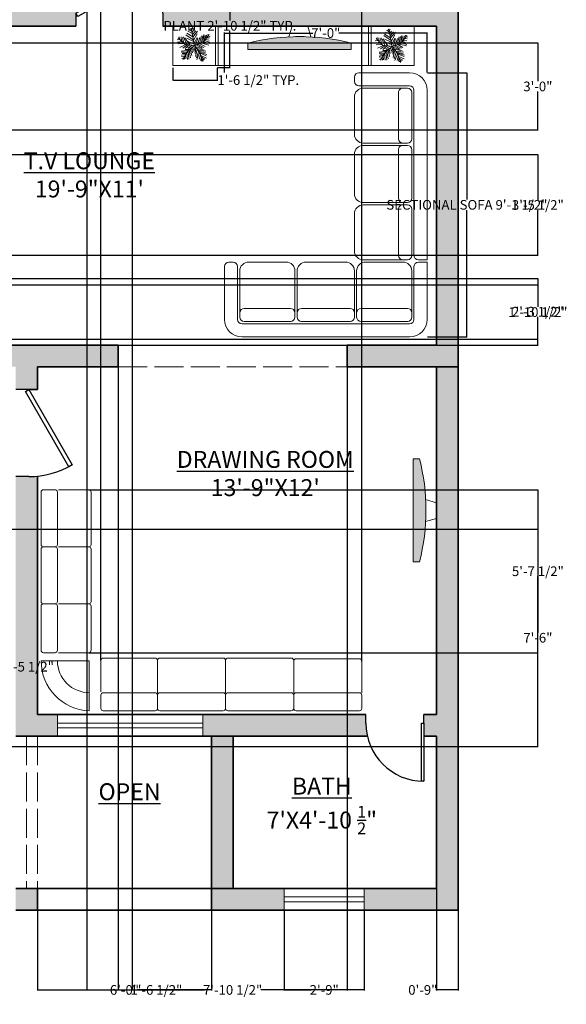
# Model space of a CAD drawing. Units: inches. Extents: x -37 to 408, y -619 to 75.
# Tile 3 of 4: x 182 to 408, y -619 to -212. Entities that reach past the tile are written whole.
import ezdxf

# ---------------------------------------------------------------- set-up
doc = ezdxf.new("R2010")
doc.units = ezdxf.units.IN
doc.header["$MEASUREMENT"] = 0
doc.linetypes.add('ACAD_ISO02W100', pattern=[15, 12, -3])
for name, color, linetype, lineweight in [('A-ANNO-DIMS', 2, 'Continuous', 18), ('A-AREA-IDEN', 7, 'Continuous', 25), ('A-DOOR', 4, 'Continuous', 25), ('A-EQPM', 9, 'Continuous', 18), ('A-FLOR-CASE', 8, 'Continuous', 18), ('A-FURN', 8, 'Continuous', 18), ('A-GLAZ', 4, 'Continuous', 18), ('A-WALL', 7, 'Continuous', 35), ('A-WALL-OVHD', 7, 'ACAD_ISO02W100', 18), ('A-WALL-PATT', 16, 'Continuous', 13), ('tree', 3, 'Continuous', 13)]:
    doc.layers.add(name, color=color, linetype=linetype, lineweight=lineweight)
doc.styles.get("Standard").update_dxf_attribs({"font": 'arial.ttf'})
doc.dimstyles.get("Standard").update_dxf_attribs({"dimtxt": 4, "dimasz": 0.18, "dimexe": 0.18, "dimexo": 0.0625, "dimgap": 0.09, "dimtad": 0, "dimtih": 1, "dimtoh": 1, "dimdec": 1, "dimzin": 0, "dimdsep": 46, "dimlunit": 4, "dimtxsty": 'Standard', "dimcen": 0.09, "dimadec": 0, "dimazin": 0, "dimtfac": 1, "dimtdec": 1, "dimtofl": 0, "dimtmove": 0, "dimatfit": 3, "dimfxl": 1, "dimtolj": 1, "dimtzin": 0, "dimarcsym": 0})

# ---------------------------------------------------------------- blocks, each defined once
blk = doc.blocks.new('*U2')
for p, q in [((0, 0), (0, -6)), ((40, 0), (40, -6))]:
    blk.add_line(p, q)
blk.add_lwpolyline([(0, 0), (34.64, 20), (35.52, 18.48), (0.87, -1.52)], close=True)
blk.add_arc((0, 0), 40, 0, 30)
blk = doc.blocks.new('*U3')
for p, q in [((0, 0), (0, -6)), ((40, 0), (40, -6))]:
    blk.add_line(p, q)
blk.add_lwpolyline([(0, 0), (0, 40), (1.75, 40), (1.75, 0)], close=True)
blk.add_arc((0, 0), 40, 0, 90)
blk = doc.blocks.new('A$C2AFA021D')
for p, q in [((0.8, 2.3), (0.2, 2.3)), ((0.85, 2.2), (0.85, 2.25)), ((0.2, 2.15), (0.8, 2.15)), ((0.225, 2.125), (0.275, 2.125)), ((0.75, 2.125), (0.275, 2.125)), ((0, 2.1), (0, 0.2)), ((0.15, 0.2), (0.15, 2.1)), ((0.175, 1.55), (0.175, 2.075)), ((0.325, 2.075), (0.325, 1.55)), ((0.85, 1.6), (0.85, 2.025)), ((0.275, 1.5), (0.225, 1.5)), ((0.225, 1.475), (0.275, 1.475)), ((0.275, 1.5), (0.75, 1.5)), ((0.75, 1.475), (0.275, 1.475)), ((0.175, 0.875), (0.175, 1.425)), ((0.325, 1.425), (0.325, 0.875)), ((0.85, 0.925), (0.85, 1.375)), ((0.275, 0.825), (0.225, 0.825)), ((0.225, 0.8), (0.275, 0.8)), ((0.275, 0.825), (0.75, 0.825)), ((0.75, 0.8), (0.275, 0.8)), ((0.975, 0.825), (1.4, 0.825)), ((1.625, 0.825), (2.075, 0.825)), ((2.3, 0.825), (2.725, 0.825)), ((2.9, 0.825), (2.95, 0.825)), ((0.175, 0.225), (0.175, 0.75)), ((0.325, 0.75), (0.325, 0.225)), ((0.85, 0.275), (0.85, 0.7)), ((0.875, 0.275), (0.875, 0.725)), ((1.5, 0.725), (1.5, 0.275)), ((1.525, 0.275), (1.525, 0.725)), ((2.175, 0.725), (2.175, 0.275)), ((2.2, 0.275), (2.2, 0.725)), ((2.825, 0.725), (2.825, 0.275)), ((2.85, 0.2), (2.85, 0.775)), ((3, 0.775), (3, 0.2)), ((0.875, 0.275), (0.875, 0.225)), ((1.45, 0.325), (0.925, 0.325)), ((1.5, 0.225), (1.5, 0.275)), ((1.525, 0.275), (1.525, 0.225)), ((2.125, 0.325), (1.575, 0.325)), ((2.175, 0.225), (2.175, 0.275)), ((2.2, 0.275), (2.2, 0.225)), ((2.775, 0.325), (2.25, 0.325)), ((2.825, 0.225), (2.825, 0.275)), ((0.8, 0.15), (0.2, 0.15)), ((0.275, 0.175), (0.225, 0.175)), ((0.275, 0.175), (0.75, 0.175)), ((0.925, 0.175), (1.45, 0.175)), ((0.925, 0.15), (2.8, 0.15)), ((1.575, 0.175), (2.125, 0.175)), ((2.25, 0.175), (2.775, 0.175)), ((0.85, 0), (0.85, 0.1)), ((0.875, 0.1), (0.875, 0)), ((0.2, 0), (0.85, 0)), ((2.8, 0), (0.875, 0))]:
    blk.add_line(p, q)
for centre, radius, start, end in [((0.2, 2.1), 0.2, 90, 180), ((0.8, 2.25), 0.05, 0, 90), ((0.2, 2.1), 0.05, 90, 180), ((0.225, 2.075), 0.05, 90, 180), ((0.275, 2.075), 0.05, 0, 90), ((0.75, 2.025), 0.1, 0, 90), ((0.8, 2.2), 0.05, 270, 0), ((0.75, 1.6), 0.1, 270, 0), ((0.225, 1.55), 0.05, 180, 270), ((0.225, 1.425), 0.05, 90, 180), ((0.275, 1.55), 0.05, 270, 0), ((0.275, 1.425), 0.05, 0, 90), ((0.75, 1.375), 0.1, 360, 90), ((0.75, 0.925), 0.1, 270, 0), ((0.225, 0.875), 0.05, 180, 270), ((0.225, 0.75), 0.05, 90, 180), ((0.275, 0.875), 0.05, 270, 0), ((0.275, 0.75), 0.05, 0, 90), ((0.75, 0.7), 0.1, 0, 90), ((0.975, 0.725), 0.1, 90, 180), ((1.4, 0.725), 0.1, 0, 90), ((1.625, 0.725), 0.1, 90, 180), ((2.075, 0.725), 0.1, 0, 90), ((2.3, 0.725), 0.1, 90, 180), ((2.725, 0.725), 0.1, 0, 90), ((2.9, 0.775), 0.05, 90, 180), ((2.95, 0.775), 0.05, 0, 90), ((0.225, 0.225), 0.05, 180, 270), ((0.275, 0.225), 0.05, 270, 0), ((0.75, 0.275), 0.1, 270, 0), ((0.925, 0.275), 0.05, 90, 180), ((0.925, 0.225), 0.05, 180, 270), ((1.45, 0.275), 0.05, 360, 90), ((1.45, 0.225), 0.05, 270, 0), ((1.575, 0.275), 0.05, 90, 180), ((1.575, 0.225), 0.05, 180, 270), ((2.125, 0.275), 0.05, 360, 90), ((2.125, 0.225), 0.05, 270, 0), ((2.25, 0.275), 0.05, 90, 180), ((2.25, 0.225), 0.05, 180, 270), ((2.775, 0.275), 0.05, 360, 90), ((2.775, 0.225), 0.05, 270, 0), ((0.2, 0.2), 0.2, 180, 270), ((0.2, 0.2), 0.05, 180, 270), ((0.8, 0.1), 0.05, 0, 90), ((0.925, 0.1), 0.05, 90, 180), ((2.8, 0.2), 0.2, 270, 0), ((2.8, 0.2), 0.05, 270, 0)]:
    blk.add_arc(centre, radius, start, end)
blk = doc.blocks.new('Trees - Imperial')
for p, q in [((-3.665, 19.273), (-27.574, 35.527)), ((-5.114, 28.097), (-24.676, 40.636)), ((-7.288, 39.707), (-21.778, 46.673)), ((-8.737, 47.138), (-17.069, 52.711)), ((-10.186, 53.64), (-13.084, 55.962)), ((0, 0), (-10.5, 57)), ((-9.099, 51.782), (-6.563, 55.962)), ((-7.65, 43.423), (-2.578, 49.46)), ((-5.839, 35.992), (4.667, 48.067)), ((-5.114, 27.632), (10.463, 46.673)), ((-2.941, 16.486), (8.652, 37.85)), ((22.055, 7.198), (27.489, 32.277)), ((27, 9), (48, 36)), ((27.127, 9.056), (31.112, 35.992)), ((35.096, 32.741), (37.27, 22.524)), ((38.719, 34.134), (41.979, 28.561)), ((44.153, 36.456), (45.239, 32.741)), ((-47.498, 19.737), (-55.83, 18.344)), ((-40.615, 13.7), (-55.105, 10.913)), ((-31.5, 4.5), (-52.5, 25.5)), ((-33.37, 6.269), (-52.207, 5.34)), ((-48.585, 21.131), (-49.309, 29.026)), ((-28.299, 3.483), (-47.86, -5.805)), ((-43.513, 28.561), (-42.427, 15.558)), ((-38.442, 26.239), (-34.819, 7.663)), ((-21.416, 3.018), (-38.079, -8.128)), ((-35.544, 28.097), (-24.314, 3.947)), ((0, 0), (-31.5, 4.5)), ((-14.533, 2.09), (-30.834, 25.31)), ((-15.982, 2.09), (-30.11, -9.521)), ((-24.314, 23.917), (-2.941, 13.7)), ((0, 0), (-22.5, -19.5)), ((-6.563, 1.161), (-21.416, -8.128)), ((-20.691, 13.7), (-1.129, 4.876)), ((-1.129, 6.734), (9.014, 26.704)), ((0, 0), (27, 9)), ((0, 0), (18, -22.5)), ((3.942, 1.625), (11.187, 24.381)), ((6.478, 1.625), (26.04, -8.592)), ((10.101, 3.483), (17.708, 26.239)), ((11.187, 3.483), (30.749, -5.805)), ((16.259, 5.805), (23.142, 31.348)), ((18.07, 5.805), (35.096, -3.483)), ((24.229, 7.663), (46.688, 1.625)), ((29.662, 12.307), (48.137, 6.269)), ((31.836, 30.883), (32.561, 16.486)), ((33.285, 16.486), (48.862, 10.913)), ((36.183, 19.737), (48.137, 17.88)), ((40.53, 25.775), (48.862, 24.846)), ((43.791, 29.954), (51.036, 30.883)), ((-17.431, -15.094), (-42.789, -18.809)), ((-28.299, -29.026), (-42.789, -31.348)), ((-24.314, -21.596), (-42.427, -22.06)), ((-26.849, -26.24), (-40.253, -25.775)), ((-22.5, -19.5), (-37.5, -45)), ((-15.257, -12.772), (-30.11, -12.772)), ((-29.023, -30.884), (-27.936, -43.887)), ((-25.038, -23.918), (-22.865, -45.281)), ((-20.691, -18.345), (-17.793, -44.352)), ((-6.563, -5.805), (-19.967, -9.985)), ((-17.069, -15.094), (-12.721, -40.172)), ((-13.446, -11.378), (-8.737, -32.741)), ((-9.461, -8.592), (-6.201, -23.453)), ((-4.752, -3.483), (-3.665, -14.629)), ((2.493, -3.019), (-1.491, -20.202)), ((1.769, -2.555), (24.229, -9.521)), ((5.029, -6.27), (2.131, -25.775)), ((9.014, -11.378), (3.58, -35.992)), ((14.085, -16.951), (6.478, -40.172)), ((7.565, -9.056), (32.198, -14.629)), ((18.07, -22.524), (8.289, -45.745)), ((12.274, -15.094), (36.907, -18.809)), ((20.244, -30.419), (15.897, -44.816)), ((16.259, -19.738), (36.183, -22.989)), ((18, -22.5), (27, -52.5)), ((18.433, -22.524), (40.53, -29.026)), ((19.157, -25.311), (38.719, -33.206)), ((-30.834, -34.135), (-42.427, -35.528)), ((-34.457, -39.708), (-40.978, -42.494)), ((-32.646, -36.921), (-31.921, -44.352)), ((22.78, -37.85), (19.519, -48.532)), ((21.331, -32.741), (39.081, -40.636)), ((22.78, -38.314), (34.372, -44.816)), ((24.591, -45.745), (23.142, -50.854)), ((24.591, -43.423), (30.749, -47.603)), ((26.764, -49.925), (28.213, -50.854))]:
    blk.add_line(p, q)
blk = doc.blocks.new('TV-WALL-MOUNT')
h = blk.add_hatch(color=256)
h.dxf.hatch_style = 1
h.set_gradient(color1=(255, 255, 255), color2=(0, 255, 255), tint=1, name='CYLINDER')
h.paths.add_polyline_path([(21.48, 5.31), (21.22, 5.31, 0.06152), (0, 2.65), (0, 0), (21.35, 0), (42.7, 0), (42.7, 2.65, 0.06152)])
for p, q in [((18.26, 9.61), (16.92, 5.19)), ((24.71, 9.61), (26.04, 5.19)), ((23.28, 5.31), (19.68, 5.31)), ((0, 2.65), (0, 0)), ((0, 0), (21.35, 0)), ((42.7, 0), (21.35, 0)), ((42.7, 2.65), (42.7, 0))]:
    blk.add_line(p, q)
blk.add_arc((21.35, -81.94), 87.25, 75.8341, 104.1659)
blk = doc.blocks.new('*D14')
at = {"layer": 'A-ANNO-DIMS', "color": 0, "lineweight": -2, "transparency": 16777216}
for p, q in [((264.05, -196.9), (269.35, -196.9)), ((269.17, -197.08), (269.17, -212.04)), ((269.17, -231.31), (269.17, -216.35)), ((264.05, -231.49), (269.35, -231.49))]:
    blk.add_line(p, q, dxfattribs=at)
at = {"layer": 'A-ANNO-DIMS', "color": 0, "transparency": 16777216}
for points in [[(269.14, -197.08), (269.2, -197.08), (269.17, -196.9)], [(269.14, -231.31), (269.2, -231.31), (269.17, -231.49)]]:
    blk.add_solid(points, dxfattribs=at)
at = {"layer": 'Defpoints', "color": 0, "transparency": 16777216}
for p in [(263.98, -196.9), (269.17, -196.9), (263.98, -231.49)]:
    blk.add_point(p, dxfattribs=at)
at = {"layer": 'A-ANNO-DIMS', "color": 0, "transparency": 16777216, "insert": (269.17, -214.2), "char_height": 4, "attachment_point": 5}
blk.add_mtext('\\A1;PLANT 2\'-10 1/2" TYP.', dxfattribs=at)
blk = doc.blocks.new('*D15')
at = {"layer": 'A-ANNO-DIMS', "color": 0, "lineweight": -2, "transparency": 16777216}
for p, q in [((245.62, -231.56), (245.62, -236.86)), ((263.98, -231.56), (263.98, -236.86)), ((245.8, -236.68), (263.8, -236.68)), ((263.98, -236.68), (264.16, -236.68))]:
    blk.add_line(p, q, dxfattribs=at)
at = {"layer": 'A-ANNO-DIMS', "color": 0, "transparency": 16777216}
for points in [[(245.8, -236.65), (245.8, -236.71), (245.62, -236.68)], [(263.8, -236.65), (263.8, -236.71), (263.98, -236.68)]]:
    blk.add_solid(points, dxfattribs=at)
at = {"layer": 'Defpoints', "color": 0, "transparency": 16777216}
for p in [(245.62, -231.49), (263.98, -231.49), (263.98, -236.68)]:
    blk.add_point(p, dxfattribs=at)
at = {"layer": 'A-ANNO-DIMS', "color": 0, "transparency": 16777216, "insert": (280.92, -236.68), "char_height": 4, "attachment_point": 5}
blk.add_mtext('\\A1;1\'-6 1/2" TYP.', dxfattribs=at)
blk = doc.blocks.new('*D24')
at = {"layer": 'A-ANNO-DIMS', "color": 0, "lineweight": -2, "transparency": 16777216}
for p, q in [((154.24, -398.74), (178.6, -398.74)), ((178.42, -398.92), (178.42, -477.4)), ((178.42, -560.19), (178.42, -481.72)), ((154.24, -560.37), (178.6, -560.37))]:
    blk.add_line(p, q, dxfattribs=at)
at = {"layer": 'A-ANNO-DIMS', "color": 0, "transparency": 16777216}
for points in [[(178.39, -398.92), (178.45, -398.92), (178.42, -398.74)], [(178.39, -560.19), (178.45, -560.19), (178.42, -560.37)]]:
    blk.add_solid(points, dxfattribs=at)
at = {"layer": 'Defpoints', "color": 0, "transparency": 16777216}
for p in [(154.18, -398.74), (154.18, -560.37), (178.42, -560.37)]:
    blk.add_point(p, dxfattribs=at)
at = {"layer": 'A-ANNO-DIMS', "color": 0, "transparency": 16777216, "insert": (178.42, -479.56), "char_height": 4, "attachment_point": 5}
blk.add_mtext('\\A1;CAR 13\'-5 1/2"', dxfattribs=at)
blk = doc.blocks.new('*D26')
at = {"layer": 'A-ANNO-DIMS', "color": 0, "lineweight": -2, "transparency": 16777216}
for p, q in [((350.87, -233.61), (367.4, -233.61)), ((367.22, -233.79), (367.22, -286.17)), ((367.22, -342.87), (367.22, -290.49)), ((350.87, -343.05), (367.4, -343.05))]:
    blk.add_line(p, q, dxfattribs=at)
at = {"layer": 'A-ANNO-DIMS', "color": 0, "transparency": 16777216}
for points in [[(367.19, -233.79), (367.25, -233.79), (367.22, -233.61)], [(367.19, -342.87), (367.25, -342.87), (367.22, -343.05)]]:
    blk.add_solid(points, dxfattribs=at)
at = {"layer": 'Defpoints', "color": 0, "transparency": 16777216}
for p in [(350.81, -233.61), (367.22, -233.61), (350.81, -343.05)]:
    blk.add_point(p, dxfattribs=at)
at = {"layer": 'A-ANNO-DIMS', "color": 0, "transparency": 16777216, "insert": (367.22, -288.33), "char_height": 4, "attachment_point": 5}
blk.add_mtext('\\A1;SECTIONAL SOFA 9\'-1 1/2"', dxfattribs=at)
blk = doc.blocks.new('*D27')
at = {"layer": 'A-ANNO-DIMS', "color": 0, "lineweight": -2, "transparency": 16777216}
for p, q in [((266.9, -233.55), (266.9, -217.01)), ((267.08, -217.19), (303.47, -217.19)), ((350.63, -217.19), (314.25, -217.19)), ((350.81, -233.55), (350.81, -217.01))]:
    blk.add_line(p, q, dxfattribs=at)
at = {"layer": 'A-ANNO-DIMS', "color": 0, "transparency": 16777216}
for points in [[(267.08, -217.16), (267.08, -217.22), (266.9, -217.19)], [(350.63, -217.16), (350.63, -217.22), (350.81, -217.19)]]:
    blk.add_solid(points, dxfattribs=at)
at = {"layer": 'Defpoints', "color": 0, "transparency": 16777216}
for p in [(266.9, -217.19), (266.9, -233.61), (350.81, -233.61)]:
    blk.add_point(p, dxfattribs=at)
at = {"layer": 'A-ANNO-DIMS', "color": 0, "transparency": 16777216, "insert": (308.86, -217.19), "char_height": 4, "attachment_point": 5}
blk.add_mtext('\\A1;7\'-0"', dxfattribs=at)
blk = doc.blocks.new('*D31')
at = {"layer": 'A-ANNO-DIMS', "color": 0, "lineweight": -2, "transparency": 16777216}
for p, q in [((189.58, -571.44), (189.58, -613.56)), ((261.58, -580.44), (261.58, -613.56)), ((189.76, -613.38), (220.16, -613.38)), ((261.4, -613.38), (231, -613.38))]:
    blk.add_line(p, q, dxfattribs=at)
at = {"layer": 'A-ANNO-DIMS', "color": 0, "transparency": 16777216}
for points in [[(189.76, -613.35), (189.76, -613.41), (189.58, -613.38)], [(261.4, -613.35), (261.4, -613.41), (261.58, -613.38)]]:
    blk.add_solid(points, dxfattribs=at)
at = {"layer": 'Defpoints', "color": 0, "transparency": 16777216}
for p in [(189.58, -571.38), (261.58, -580.38), (261.58, -613.38)]:
    blk.add_point(p, dxfattribs=at)
at = {"layer": 'A-ANNO-DIMS', "color": 0, "transparency": 16777216, "insert": (225.58, -613.38), "char_height": 4, "attachment_point": 5}
blk.add_mtext('\\A1;6\'-0"', dxfattribs=at)
blk = doc.blocks.new('*D35')
at = {"layer": 'A-ANNO-DIMS', "color": 0, "lineweight": -2, "transparency": 16777216}
for p, q in [((222.97, -355.44), (222.97, -613.56)), ((317.68, -355.44), (317.68, -613.56)), ((223.15, -613.38), (258.72, -613.38)), ((317.5, -613.38), (281.93, -613.38))]:
    blk.add_line(p, q, dxfattribs=at)
at = {"layer": 'A-ANNO-DIMS', "color": 0, "transparency": 16777216}
for points in [[(223.15, -613.35), (223.15, -613.41), (222.97, -613.38)], [(317.5, -613.35), (317.5, -613.41), (317.68, -613.38)]]:
    blk.add_solid(points, dxfattribs=at)
at = {"layer": 'Defpoints', "color": 0, "transparency": 16777216}
for p in [(222.97, -355.38), (317.68, -355.38), (317.68, -613.38)]:
    blk.add_point(p, dxfattribs=at)
at = {"layer": 'A-ANNO-DIMS', "color": 0, "transparency": 16777216, "insert": (270.32, -613.38), "char_height": 4, "attachment_point": 5}
blk.add_mtext('\\A1;7\'-10 1/2"', dxfattribs=at)
blk = doc.blocks.new('*D40')
at = {"layer": 'A-ANNO-DIMS', "color": 0, "lineweight": -2, "transparency": 16777216}
for p, q in [((354.58, -571.44), (354.58, -613.56)), ((363.58, -580.44), (363.58, -613.56)), ((354.58, -613.38), (354.4, -613.38)), ((363.4, -613.38), (354.76, -613.38))]:
    blk.add_line(p, q, dxfattribs=at)
at = {"layer": 'A-ANNO-DIMS', "color": 0, "transparency": 16777216}
for points in [[(354.76, -613.35), (354.76, -613.41), (354.58, -613.38)], [(363.4, -613.35), (363.4, -613.41), (363.58, -613.38)]]:
    blk.add_solid(points, dxfattribs=at)
at = {"layer": 'Defpoints', "color": 0, "transparency": 16777216}
for p in [(354.58, -571.38), (363.58, -580.38), (354.58, -613.38)]:
    blk.add_point(p, dxfattribs=at)
at = {"layer": 'A-ANNO-DIMS', "color": 0, "transparency": 16777216, "insert": (348.99, -613.38), "char_height": 4, "attachment_point": 5}
blk.add_mtext('\\A1;0\'-9"', dxfattribs=at)
blk = doc.blocks.new('*D42')
at = {"layer": 'A-ANNO-DIMS', "color": 0, "lineweight": -2, "transparency": 16777216}
for p, q in [((48.64, -422.57), (396.76, -422.57)), ((396.58, -422.75), (396.58, -465.43)), ((396.58, -512.39), (396.58, -469.7)), ((48.64, -512.57), (396.76, -512.57))]:
    blk.add_line(p, q, dxfattribs=at)
at = {"layer": 'A-ANNO-DIMS', "color": 0, "transparency": 16777216}
for points in [[(396.55, -422.75), (396.61, -422.75), (396.58, -422.57)], [(396.55, -512.39), (396.61, -512.39), (396.58, -512.57)]]:
    blk.add_solid(points, dxfattribs=at)
at = {"layer": 'Defpoints', "color": 0, "transparency": 16777216}
for p in [(48.58, -422.57), (396.58, -422.57), (48.58, -512.57)]:
    blk.add_point(p, dxfattribs=at)
at = {"layer": 'A-ANNO-DIMS', "color": 0, "transparency": 16777216, "insert": (396.58, -467.57), "char_height": 4, "attachment_point": 5}
blk.add_mtext('\\A1;7\'-6"', dxfattribs=at)
blk = doc.blocks.new('*D44')
at = {"layer": 'A-ANNO-DIMS', "color": 0, "lineweight": -2, "transparency": 16777216}
for p, q in [((89.6, -321.48), (396.76, -321.48)), ((396.58, -321.66), (396.58, -330.57)), ((396.58, -343.8), (396.58, -334.89)), ((89.76, -343.98), (396.76, -343.98))]:
    blk.add_line(p, q, dxfattribs=at)
at = {"layer": 'A-ANNO-DIMS', "color": 0, "transparency": 16777216}
for points in [[(396.55, -321.66), (396.61, -321.66), (396.58, -321.48)], [(396.55, -343.8), (396.61, -343.8), (396.58, -343.98)]]:
    blk.add_solid(points, dxfattribs=at)
at = {"layer": 'Defpoints', "color": 0, "transparency": 16777216}
for p in [(89.54, -321.48), (396.58, -321.48), (89.69, -343.98)]:
    blk.add_point(p, dxfattribs=at)
at = {"layer": 'A-ANNO-DIMS', "color": 0, "transparency": 16777216, "insert": (396.58, -332.73), "char_height": 4, "attachment_point": 5}
blk.add_mtext('\\A1;1\'-10 1/2"', dxfattribs=at)
blk = doc.blocks.new('*D45')
at = {"layer": 'A-ANNO-DIMS', "color": 0, "lineweight": -2, "transparency": 16777216}
for p, q in [((117.64, -221.31), (396.76, -221.31)), ((396.58, -221.49), (396.58, -237.17)), ((396.58, -257.13), (396.58, -241.44)), ((117.64, -257.31), (396.76, -257.31))]:
    blk.add_line(p, q, dxfattribs=at)
at = {"layer": 'A-ANNO-DIMS', "color": 0, "transparency": 16777216}
for points in [[(396.55, -221.49), (396.61, -221.49), (396.58, -221.31)], [(396.55, -257.13), (396.61, -257.13), (396.58, -257.31)]]:
    blk.add_solid(points, dxfattribs=at)
at = {"layer": 'Defpoints', "color": 0, "transparency": 16777216}
for p in [(117.58, -221.31), (396.58, -221.31), (117.58, -257.31)]:
    blk.add_point(p, dxfattribs=at)
at = {"layer": 'A-ANNO-DIMS', "color": 0, "transparency": 16777216, "insert": (396.58, -239.31), "char_height": 4, "attachment_point": 5}
blk.add_mtext('\\A1;3\'-0"', dxfattribs=at)
blk = doc.blocks.new('*D46')
at = {"layer": 'A-ANNO-DIMS', "color": 0, "lineweight": -2, "transparency": 16777216}
for p, q in [((108.64, -318.81), (396.76, -318.81)), ((396.58, -318.99), (396.58, -330.43)), ((396.58, -346.2), (396.58, -334.75)), ((108.64, -346.38), (396.76, -346.38))]:
    blk.add_line(p, q, dxfattribs=at)
at = {"layer": 'A-ANNO-DIMS', "color": 0, "transparency": 16777216}
for points in [[(396.55, -318.99), (396.61, -318.99), (396.58, -318.81)], [(396.55, -346.2), (396.61, -346.2), (396.58, -346.38)]]:
    blk.add_solid(points, dxfattribs=at)
at = {"layer": 'Defpoints', "color": 0, "transparency": 16777216}
for p in [(108.58, -318.81), (108.58, -346.38), (396.58, -346.38)]:
    blk.add_point(p, dxfattribs=at)
at = {"layer": 'A-ANNO-DIMS', "color": 0, "transparency": 16777216, "insert": (396.58, -332.59), "char_height": 4, "attachment_point": 5}
blk.add_mtext('\\A1;2\'-3 1/2"', dxfattribs=at)
blk = doc.blocks.new('*D48')
at = {"layer": 'A-ANNO-DIMS', "color": 0, "lineweight": -2, "transparency": 16777216}
for p, q in [((209.99, -49.44), (209.99, -613.56)), ((228.72, -49.44), (228.72, -613.56)), ((210.17, -613.38), (228.54, -613.38)), ((228.72, -613.38), (228.9, -613.38))]:
    blk.add_line(p, q, dxfattribs=at)
at = {"layer": 'A-ANNO-DIMS', "color": 0, "transparency": 16777216}
for points in [[(210.17, -613.35), (210.17, -613.41), (209.99, -613.38)], [(228.54, -613.35), (228.54, -613.41), (228.72, -613.38)]]:
    blk.add_solid(points, dxfattribs=at)
at = {"layer": 'Defpoints', "color": 0, "transparency": 16777216}
for p in [(209.99, -49.38), (228.72, -49.38), (228.72, -613.38)]:
    blk.add_point(p, dxfattribs=at)
at = {"layer": 'A-ANNO-DIMS', "color": 0, "transparency": 16777216, "insert": (238.78, -613.38), "char_height": 4, "attachment_point": 5}
blk.add_mtext('\\A1;1\'-6 1/2"', dxfattribs=at)
blk = doc.blocks.new('*D49')
at = {"layer": 'A-ANNO-DIMS', "color": 0, "lineweight": -2, "transparency": 16777216}
for p, q in [((291.68, -580.44), (291.68, -613.56)), ((324.75, -580.44), (324.75, -613.56)), ((291.86, -613.38), (302.77, -613.38)), ((324.57, -613.38), (313.65, -613.38))]:
    blk.add_line(p, q, dxfattribs=at)
at = {"layer": 'A-ANNO-DIMS', "color": 0, "transparency": 16777216}
for points in [[(291.86, -613.35), (291.86, -613.41), (291.68, -613.38)], [(324.57, -613.35), (324.57, -613.41), (324.75, -613.38)]]:
    blk.add_solid(points, dxfattribs=at)
at = {"layer": 'Defpoints', "color": 0, "transparency": 16777216}
for p in [(291.68, -580.38), (324.75, -580.38), (324.75, -613.38)]:
    blk.add_point(p, dxfattribs=at)
at = {"layer": 'A-ANNO-DIMS', "color": 0, "transparency": 16777216, "insert": (308.21, -613.38), "char_height": 4, "attachment_point": 5}
blk.add_mtext('\\A1;2\'-9"', dxfattribs=at)
blk = doc.blocks.new('*D50')
at = {"layer": 'A-ANNO-DIMS', "color": 0, "lineweight": -2, "transparency": 16777216}
for p, q in [((215.83, -476.93), (215.83, 69.37)), ((323.75, -477.22), (323.75, 69.37)), ((216.01, 69.19), (264.38, 69.19)), ((323.57, 69.19), (275.2, 69.19))]:
    blk.add_line(p, q, dxfattribs=at)
at = {"layer": 'A-ANNO-DIMS', "color": 0, "transparency": 16777216}
for points in [[(216.01, 69.22), (216.01, 69.16), (215.83, 69.19)], [(323.57, 69.22), (323.57, 69.16), (323.75, 69.19)]]:
    blk.add_solid(points, dxfattribs=at)
at = {"layer": 'Defpoints', "color": 0, "transparency": 16777216}
for p in [(323.75, 69.19), (215.83, -476.99), (323.75, -477.28)]:
    blk.add_point(p, dxfattribs=at)
at = {"layer": 'A-ANNO-DIMS', "color": 0, "transparency": 16777216, "insert": (269.79, 69.19), "char_height": 4, "attachment_point": 5}
blk.add_mtext('\\A1;9\'-0"', dxfattribs=at)
blk = doc.blocks.new('*D51')
at = {"layer": 'A-ANNO-DIMS', "color": 0, "lineweight": -2, "transparency": 16777216}
for p, q in [((210.87, -406.31), (396.76, -406.31)), ((396.58, -406.49), (396.58, -437.88)), ((396.58, -473.58), (396.58, -442.19)), ((210.87, -473.76), (396.76, -473.76))]:
    blk.add_line(p, q, dxfattribs=at)
at = {"layer": 'A-ANNO-DIMS', "color": 0, "transparency": 16777216}
for points in [[(396.55, -406.49), (396.61, -406.49), (396.58, -406.31)], [(396.55, -473.58), (396.61, -473.58), (396.58, -473.76)]]:
    blk.add_solid(points, dxfattribs=at)
at = {"layer": 'Defpoints', "color": 0, "transparency": 16777216}
for p in [(210.8, -406.31), (396.58, -406.31), (210.8, -473.76)]:
    blk.add_point(p, dxfattribs=at)
at = {"layer": 'A-ANNO-DIMS', "color": 0, "transparency": 16777216, "insert": (396.58, -440.04), "char_height": 4, "attachment_point": 5}
blk.add_mtext('\\A1;5\'-7 1/2"', dxfattribs=at)
blk = doc.blocks.new('*D52')
at = {"layer": 'A-ANNO-DIMS', "color": 0, "lineweight": -2, "transparency": 16777216}
for p, q in [((126.12, -267.56), (396.76, -267.56)), ((396.58, -267.74), (396.58, -286.24)), ((396.58, -309.05), (396.58, -290.56)), ((126.12, -309.23), (396.76, -309.23))]:
    blk.add_line(p, q, dxfattribs=at)
at = {"layer": 'A-ANNO-DIMS', "color": 0, "transparency": 16777216}
for points in [[(396.55, -267.74), (396.61, -267.74), (396.58, -267.56)], [(396.55, -309.05), (396.61, -309.05), (396.58, -309.23)]]:
    blk.add_solid(points, dxfattribs=at)
at = {"layer": 'Defpoints', "color": 0, "transparency": 16777216}
for p in [(126.06, -267.56), (126.06, -309.23), (396.58, -309.23)]:
    blk.add_point(p, dxfattribs=at)
at = {"layer": 'A-ANNO-DIMS', "color": 0, "transparency": 16777216, "insert": (396.58, -288.4), "char_height": 4, "attachment_point": 5}
blk.add_mtext('\\A1;3\'-5 1/2"', dxfattribs=at)

msp = doc.modelspace()

# ---------------------------------------------------------------- hatches: boundary and pattern name
at = {"layer": 'A-WALL-PATT'}
h = msp.add_hatch(color=256, dxfattribs=at)
h.dxf.hatch_style = 1
h.paths.add_polyline_path([(117.58, 28.62), (3.58, 28.62), (3.58, -49.38), (19.34, -49.38), (19.34, -45.78), (19.34, -44.88), (12.58, -44.88), (12.58, 19.62), (108.58, 19.62), (108.58, 5.94), (117.58, 5.94), (117.58, 19.62)])
h.paths.add_polyline_path([(363.58, 28.62), (261.58, 28.62), (261.58, 19.62), (261.58, 6.04), (265.18, 6.04, -0.056797), (270.58, 5.42), (270.58, 19.62), (354.58, 19.62), (354.58, -44.88), (363.58, -44.88)])
h.paths.add_polyline_path([(124.92, -40.38), (117.58, -40.38), (117.58, -20.71), (108.58, -20.71), (108.58, -44.88), (43.33, -44.88, -0.009377), (43.34, -45.78), (43.34, -49.38), (124.92, -49.38)])
h.paths.add_polyline_path([(209.99, -40.38), (164.76, -40.38), (164.76, -49.38), (209.99, -49.38)])
h.paths.add_polyline_path([(270.58, -17.96), (265.18, -17.96), (261.58, -17.96), (261.58, -40.38), (252.1, -40.38, -0.056797), (252.72, -45.78), (252.72, -49.38), (354.58, -49.38), (354.58, -205.38), (363.58, -205.38), (363.58, -44.88), (354.58, -44.88), (270.58, -44.88)])
h.paths.add_polyline_path([(12.58, -49.38), (3.58, -49.38), (3.58, -205.38), (12.58, -205.38)])
h.paths.add_polyline_path([(205.47, -208.98), (205.47, -205.38), (159.34, -205.38), (159.34, -208.98), (159.34, -214.38), (205.47, -214.38)])
h = msp.add_hatch(color=256, dxfattribs=at)
h.dxf.hatch_style = 1
h.paths.add_polyline_path([(123.52, -205.38), (3.58, -205.38), (3.58, -355.38), (27.35, -355.38), (27.35, -346.38), (12.58, -346.38), (12.58, -214.38), (123.34, -214.38), (123.34, -208.98, -0.025047)])
h.paths.add_polyline_path([(117.58, -214.38), (108.58, -214.38), (108.58, -221.31), (112.18, -221.31), (117.58, -221.31)], flags=17)
h.paths.add_polyline_path([(124.36, -346.38), (86.98, -346.38), (86.98, -355.38), (124.36, -355.38), (124.36, -351.78)])
h.paths.add_polyline_path([(222.97, -346.38), (172.36, -346.38), (172.36, -351.78), (172.36, -355.38), (180.58, -355.38), (180.58, -364.83), (185.98, -364.83), (189.58, -364.83), (189.58, -355.38), (222.97, -355.38)])
h.paths.add_polyline_path([(363.58, -205.38), (241.29, -205.38, -0.025047), (241.47, -208.98), (241.47, -214.38), (354.58, -214.38), (354.58, -346.38), (317.68, -346.38), (317.68, -355.38), (363.58, -355.38)])
h = msp.add_hatch(color=256, dxfattribs=at)
h.dxf.hatch_style = 1
h.paths.add_polyline_path([(363.58, -355.38), (354.58, -355.38), (354.58, -499.38), (349.43, -499.38), (349.43, -502.98), (349.43, -508.38), (354.58, -508.38), (354.58, -571.38), (324.75, -571.38), (324.75, -580.38), (363.58, -580.38)])
h.paths.add_polyline_path([(291.68, -571.38), (261.58, -571.38), (261.58, -580.38), (291.68, -580.38)])
h.paths.add_polyline_path([(270.58, -508.38), (261.58, -508.38), (261.58, -571.38), (270.58, -571.38)])
h.paths.add_polyline_path([(325.43, -499.38), (258.03, -499.38), (258.03, -508.38), (326.04, -508.38, -0.056797), (325.43, -502.98)])
h.paths.add_polyline_path([(189.58, -571.38), (180.58, -571.38), (180.58, -580.38), (189.58, -580.38)])
h.paths.add_polyline_path([(189.58, -400.65, -0.025047), (185.98, -400.83), (180.58, -400.83), (180.58, -508.38), (189.58, -508.38), (197.89, -508.38), (197.89, -499.38), (189.58, -499.38)])
h.paths.add_polyline_path([(66.73, -571.38), (59.87, -571.38), (59.87, -580.38), (66.73, -580.38)])
h.paths.add_polyline_path([(12.58, -355.38), (3.58, -355.38), (3.58, -580.38), (12.58, -580.38), (12.58, -571.38)])

# ---------------------------------------------------------------- linework, layer by layer
at = {"layer": 'A-FLOR-CASE'}
for p, q in [((245.53, -230.63), (245.53, -214.38)), ((263.24, -214.38), (263.24, -230.63)), ((264.3, -214.38), (264.3, -230.63)), ((326.59, -214.38), (326.59, -230.63)), ((327.65, -214.38), (327.65, -230.63)), ((345.37, -214.38), (345.37, -230.63)), ((345.37, -230.63), (245.53, -230.63))]:
    msp.add_line(p, q, dxfattribs=at)
at = {"layer": 'A-FURN'}
for p, q in [((191.1, -407.31), (191.1, -428.93)), ((192.1, -406.31), (196.87, -406.31)), ((197.87, -407.31), (197.87, -428.93)), ((198.25, -406.31), (210.8, -406.31)), ((211.8, -407.31), (211.8, -428.93)), ((191.1, -430.93), (191.1, -452.54)), ((192.1, -429.93), (196.87, -429.93)), ((197.87, -430.93), (197.87, -452.54)), ((210.8, -429.93), (198.25, -429.93)), ((211.8, -430.93), (211.8, -452.54)), ((191.1, -472.76), (191.1, -454.54)), ((192.1, -453.54), (196.87, -453.54)), ((197.87, -454.54), (197.87, -472.76)), ((210.8, -453.54), (198.25, -453.54)), ((211.8, -454.54), (211.8, -472.76)), ((192.1, -473.76), (196.87, -473.76)), ((210.8, -473.76), (198.25, -473.76)), ((216.83, -475.99), (238.22, -475.99)), ((240.22, -475.99), (266.39, -475.99)), ((268.39, -475.99), (294.57, -475.99)), ((296.57, -476.28), (322.75, -476.28)), ((197.87, -477.15), (191.1, -477.15)), ((191.1, -477.15), (197.87, -477.15)), ((197.87, -477.15), (211.04, -477.15)), ((211.04, -477.15), (211.04, -490.32)), ((215.83, -489.99), (215.83, -476.99)), ((239.22, -490.32), (239.22, -476.99)), ((267.39, -490.32), (267.39, -476.99)), ((295.57, -490.32), (295.57, -477.28)), ((323.75, -490.32), (323.75, -477.28)), ((211.04, -490.32), (211.04, -497.8)), ((211.04, -497.8), (211.04, -490.32)), ((215.83, -491.32), (215.83, -496.82)), ((216.83, -490.32), (238.22, -490.32)), ((239.22, -496.82), (239.22, -491.32)), ((240.22, -490.32), (266.39, -490.32)), ((267.39, -496.8), (267.39, -491.32)), ((268.39, -490.32), (294.57, -490.32)), ((295.57, -496.8), (295.57, -491.32)), ((322.75, -490.32), (296.57, -490.32)), ((323.75, -496.8), (323.75, -491.32)), ((216.83, -497.82), (238.22, -497.82)), ((240.22, -497.8), (266.39, -497.8)), ((268.39, -497.8), (294.57, -497.8)), ((296.57, -497.8), (322.75, -497.8))]:
    msp.add_line(p, q, dxfattribs=at)
for centre, radius, start, end in [((192.1, -407.31), 1, 90, 180), ((196.87, -407.31), 1, 0, 90), ((210.8, -407.31), 1, 360, 90), ((192.1, -428.93), 1, 180, 270), ((192.1, -430.93), 1, 90, 180), ((196.87, -428.93), 1, 270, 0), ((196.87, -430.93), 1, 0, 90), ((210.8, -428.93), 1, 270, 360), ((210.8, -430.93), 1, 360, 90), ((192.1, -452.54), 1, 180, 270), ((192.1, -454.54), 1, 90, 180), ((196.87, -452.54), 1, 270, 0), ((196.87, -454.54), 1, 0, 90), ((210.8, -452.54), 1, 270, 360), ((210.8, -454.54), 1, 360, 90), ((192.1, -472.76), 1, 180, 270), ((196.87, -472.76), 1, 270, 0), ((210.8, -472.76), 1, 270, 360), ((216.83, -476.99), 1, 90, 180), ((238.22, -476.99), 1, 0, 90), ((240.22, -476.99), 1, 90, 180), ((266.39, -476.99), 1, 0, 90), ((268.39, -476.99), 1, 90, 180), ((294.57, -476.99), 1, 0, 90), ((296.57, -477.28), 1, 90, 180), ((322.75, -477.28), 1, 0, 90), ((211.77, -477.15), 20.67, 180, 267.9675), ((211.04, -477.15), 13.17, 179.9994, 270), ((216.83, -491.32), 1, 90, 180), ((238.22, -491.32), 1, 0, 90), ((240.22, -491.32), 1, 90, 180), ((266.39, -491.32), 1, 0, 90), ((268.39, -491.32), 1, 90, 180), ((294.57, -491.32), 1, 0, 90), ((296.57, -491.32), 1, 90, 180), ((322.75, -491.32), 1, 0, 90), ((216.83, -496.82), 1, 180, 270), ((238.22, -496.82), 1, 270, 0), ((240.22, -496.8), 1, 180, 270), ((266.39, -496.8), 1, 270, 0), ((268.39, -496.8), 1, 180, 270), ((294.57, -496.8), 1, 270, 0), ((296.57, -496.8), 1, 180, 270), ((322.75, -496.8), 1, 270, 0)]:
    msp.add_arc(centre, radius, start, end, dxfattribs=at)
at = {"layer": 'A-GLAZ'}
for p, q in [((197.89, -499.38), (197.89, -508.38)), ((258.03, -499.38), (258.03, -508.38)), ((258.03, -502.88), (197.89, -502.88)), ((258.03, -504.88), (197.89, -504.88)), ((291.68, -571.38), (291.68, -580.38)), ((324.75, -580.38), (324.75, -571.38)), ((291.68, -574.88), (324.75, -574.88)), ((291.68, -576.88), (324.75, -576.88))]:
    msp.add_line(p, q, dxfattribs=at)
at = {"layer": 'A-WALL'}
for p, q in [((363.58, 28.62), (363.58, -580.38)), ((159.34, -214.38), (205.47, -214.38)), ((241.47, -214.38), (354.58, -214.38)), ((354.58, -214.38), (354.58, -346.38)), ((172.36, -346.38), (222.97, -346.38)), ((222.97, -346.38), (222.97, -355.38)), ((317.68, -346.38), (317.68, -355.38)), ((317.68, -346.38), (354.58, -346.38)), ((189.58, -355.38), (189.58, -364.83)), ((189.58, -355.38), (222.97, -355.38)), ((317.68, -355.38), (363.58, -355.38)), ((354.58, -355.38), (354.58, -499.38)), ((185.98, -364.83), (189.58, -364.83)), ((189.58, -400.65), (189.58, -499.38)), ((189.58, -499.38), (325.43, -499.38)), ((349.43, -499.38), (354.58, -499.38)), ((189.58, -508.38), (180.58, -508.38)), ((189.58, -508.38), (326.04, -508.38)), ((261.58, -508.38), (261.58, -580.38)), ((270.58, -508.38), (270.58, -571.38)), ((349.43, -508.38), (354.58, -508.38)), ((354.58, -508.38), (354.58, -571.38)), ((180.58, -571.38), (354.58, -571.38)), ((189.58, -571.38), (189.58, -580.38)), ((180.58, -580.38), (363.58, -580.38))]:
    msp.add_line(p, q, dxfattribs=at)
at = {"layer": 'A-WALL-OVHD'}
for p, q in [((222.97, -346.38), (317.68, -346.38)), ((222.97, -355.38), (317.68, -355.38)), ((185.08, -508.38), (185.08, -571.38)), ((189.58, -508.38), (189.58, -571.38))]:
    msp.add_line(p, q, dxfattribs=at)

# ---------------------------------------------------------------- block references
at = {"layer": 'A-DOOR', "xscale": 0.9, "yscale": 0.9, "zscale": 0.9}
msp.add_blockref('*U2', (205.47, -208.98), dxfattribs=at)
at = {"layer": 'A-DOOR'}
for name, p, xscale, yscale, zscale, rotation in [('*U2', (185.98, -364.83), 0.9, 0.9, 0.9, 270), ('*U3', (349.43, -502.98), 0.6, 0.6, 0.6, 180)]:
    msp.add_blockref(name, p, dxfattribs=dict(at, xscale=xscale, yscale=yscale, zscale=zscale, rotation=rotation))
at = {"layer": 'A-EQPM'}
msp.add_blockref('TV-WALL-MOUNT', (276.67, -223.99), dxfattribs=at)
at = {"layer": 'A-EQPM', "rotation": 270.0000000000002}
msp.add_blockref('TV-WALL-MOUNT', (344.97, -393.44), dxfattribs=at)
at = {"layer": 'A-FURN', "xscale": 36.47919723421842, "yscale": 36.47919723421842, "zscale": 36.47919723421842, "rotation": 90}
msp.add_blockref('A$C2AFA021D', (350.81, -343.05), dxfattribs=at)
at = {"layer": 'tree', "xscale": 0.1267004668732905, "yscale": 0.1267004668732905, "zscale": 0.1267004668732905}
for p in [(254.51, -222.39), (336.3, -222.75)]:
    msp.add_blockref('Trees - Imperial', p, dxfattribs=at)

# ---------------------------------------------------------------- texts
at = {"layer": 'A-AREA-IDEN', "char_height": 7, "attachment_point": 1}
for s, width, insert in [('\\A1;\\pxqc;{\\fArial|b1|i0|c0|p34;\\LT.V LOUNGE\\l\\P19\'-9"X11\'}', 71.4915, (175.32, -266.59)), ('\\A1;\\pxqc;{\\fArial|b1|i0|c0|p34;\\LDRAWING ROOM\\l\\P13\'-9"X12\'}', 83.6613, (241.99, -390.24)), ('\\A1;\\pxqc;{\\fArial|b1|i0|c0|p34;\\LBATH\\P\\l7\'X4\'-10 \\H0.7x;\\S1/2;\\H1.42857x;"}', 54.9946, (279.73, -525.51)), ('\\A1;\\pxqc;{\\fArial|b1|i0|c0|p34;\\LOPEN}', 57.1656, (199.1, -527.83))]:
    msp.add_mtext_dynamic_manual_height_columns(s, width=width, gutter_width=1, heights=[0], dxfattribs=dict(at, insert=insert))

# ---------------------------------------------------------------- dimensions: what is measured, and where the dimension line sits
at = {"layer": 'A-ANNO-DIMS'}
for base, p1, p2, picture, middle in [((323.75, 69.19), (215.83, -476.99), (323.75, -477.28), '*D50', (269.79, 69.19)), ((228.72, -613.38), (209.99, -49.38), (228.72, -49.38), '*D48', (238.78, -613.38)), ((317.68, -613.38), (222.97, -355.38), (317.68, -355.38), '*D35', (270.32, -613.38)), ((261.58, -613.38), (189.58, -571.38), (261.58, -580.38), '*D31', (225.58, -613.38)), ((354.58, -613.38), (363.58, -580.38), (354.58, -571.38), '*D40', (348.99, -613.38)), ((324.75, -613.38), (291.68, -580.38), (324.75, -580.38), '*D49', (308.21, -613.38))]:
    dim = msp.add_linear_dim(base=base, p1=p1, p2=p2, dimstyle='Standard', override={"dimdec": 1, "dimlfac": 1, "dimrnd": 0, "dimzin": 1, "dimdsep": 46, "dimlunit": 4, "dimfrac": 2}, dxfattribs=at)
    dim.commit()
    dim.dimension.update_dxf_attribs({"geometry": picture, "text_midpoint": middle})
for base, p1, p2, angle, text, picture, middle in [((269.17, -196.9), (263.98, -231.49), (263.98, -196.9), 90, 'PLANT <> TYP.', '*D14', (269.17, -214.2)), ((367.22, -233.61), (350.81, -343.05), (350.81, -233.61), 90, 'SECTIONAL SOFA <>', '*D26', (367.22, -288.33)), ((178.42, -560.37), (154.18, -398.74), (154.18, -560.37), 270, 'CAR <>', '*D24', (178.42, -479.56))]:
    dim = msp.add_linear_dim(base=base, p1=p1, p2=p2, angle=angle, text=text, dimstyle='Standard', override={"dimdec": 1, "dimlfac": 1, "dimrnd": 0, "dimzin": 1, "dimdsep": 46, "dimlunit": 4, "dimfrac": 2}, dxfattribs=at)
    dim.commit()
    dim.dimension.update_dxf_attribs({"geometry": picture, "text_midpoint": middle})
for base, p1, p2, angle, picture, middle in [((266.9, -217.19), (350.81, -233.61), (266.9, -233.61), 180, '*D27', (308.86, -217.19)), ((396.58, -221.31), (117.58, -257.31), (117.58, -221.31), 90, '*D45', (396.58, -239.31)), ((396.58, -309.23), (126.06, -267.56), (126.06, -309.23), 90, '*D52', (396.58, -288.4)), ((396.58, -321.48), (89.69, -343.98), (89.54, -321.48), 90, '*D44', (396.58, -332.73)), ((396.58, -346.38), (108.58, -318.81), (108.58, -346.38), 90, '*D46', (396.58, -332.59)), ((396.5782, -406.3137), (210.8027, -473.7596), (210.8027, -406.3137), 90, '*D51', (396.5782, -440.0366)), ((396.58, -422.57), (48.58, -512.57), (48.58, -422.57), 90, '*D42', (396.58, -467.57))]:
    dim = msp.add_linear_dim(base=base, p1=p1, p2=p2, angle=angle, dimstyle='Standard', override={"dimdec": 1, "dimlfac": 1, "dimrnd": 0, "dimzin": 1, "dimdsep": 46, "dimlunit": 4, "dimfrac": 2}, dxfattribs=at)
    dim.commit()
    dim.dimension.update_dxf_attribs({"geometry": picture, "text_midpoint": middle})
dim = msp.add_linear_dim(base=(263.98, -236.68), p1=(245.62, -231.49), p2=(263.98, -231.49), text='<> TYP.', dimstyle='Standard', override={"dimdec": 1, "dimlfac": 1, "dimrnd": 0, "dimzin": 1, "dimdsep": 46, "dimlunit": 4, "dimfrac": 2}, dxfattribs=at)
dim.commit()
dim.dimension.update_dxf_attribs({"geometry": '*D15', "text_midpoint": (280.92, -236.68)})

doc.saveas('drawing.dxf')
